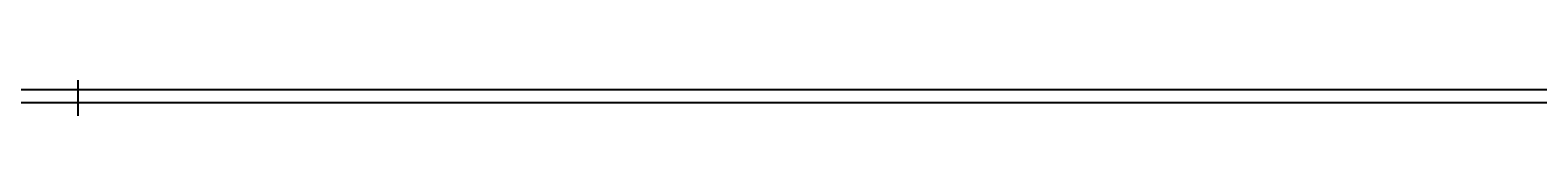
# Model space of a CAD drawing. Units: inches. Extents: x 35362 to 73946, y 43607 to 67532.
# Tile 101 of 134: x 50119 to 50761, y 49313 to 49320. Entities that reach past the tile are written whole.
import ezdxf

# ---------------------------------------------------------------- set-up
doc = ezdxf.new("R2010")
doc.units = ezdxf.units.IN
doc.header["$MEASUREMENT"] = 0
doc.layers.add('A-ANNO-DIMS', color=2, linetype='Continuous', lineweight=18)
doc.styles.get("Standard").update_dxf_attribs({"font": 'arial.ttf'})
doc.dimstyles.get("Standard").update_dxf_attribs({"dimtxt": 0.18, "dimasz": 0.18, "dimexe": 0.18, "dimexo": 0.0625, "dimgap": 0.09, "dimtad": 0, "dimtih": 1, "dimtoh": 1, "dimdec": 4, "dimzin": 0, "dimdsep": 46, "dimtxsty": 'Standard', "dimcen": 0.09, "dimadec": 0, "dimazin": 0, "dimtfac": 1, "dimtdec": 4, "dimtofl": 0, "dimtmove": 0, "dimatfit": 3, "dimfxl": 1, "dimtolj": 1, "dimtzin": 0, "dimarcsym": 0})

# ---------------------------------------------------------------- blocks, each defined once
blk = doc.blocks.new('*D11')
at = {"layer": 'A-ANNO-DIMS', "color": 0, "lineweight": -2, "transparency": 16777216}
for p, q in [((47978.66, 56028.77), (47978.66, 43606.68)), ((53109.76, 56028.77), (53109.76, 43606.68)), ((47978.84, 43606.86), (50543.87, 43606.86)), ((53109.58, 43606.86), (50544.55, 43606.86))]:
    blk.add_line(p, q, dxfattribs=at)
at = {"layer": 'A-ANNO-DIMS', "color": 0, "transparency": 16777216}
for points in [[(47978.84, 43606.89), (47978.84, 43606.83), (47978.66, 43606.86)], [(53109.58, 43606.89), (53109.58, 43606.83), (53109.76, 43606.86)]]:
    blk.add_solid(points, dxfattribs=at)
at = {"layer": 'Defpoints', "color": 0, "transparency": 16777216}
for p in [(47978.66, 56028.84), (53109.76, 56028.84), (53109.76, 43606.86)]:
    blk.add_point(p, dxfattribs=at)
at = {"layer": 'A-ANNO-DIMS', "color": 0, "transparency": 16777216, "insert": (50544.21, 43606.86), "char_height": 0.18, "attachment_point": 5}
blk.add_mtext('\\A1;5131', dxfattribs=at)
blk = doc.blocks.new('*D13')
at = {"layer": 'A-ANNO-DIMS', "color": 0, "lineweight": -2, "transparency": 16777216}
for p, q in [((48373.49, 51694.02), (48373.49, 43606.68)), ((51029.04, 51694.02), (51029.04, 43606.68)), ((48373.67, 43606.86), (49700.8, 43606.86)), ((51028.86, 43606.86), (49701.73, 43606.86))]:
    blk.add_line(p, q, dxfattribs=at)
at = {"layer": 'A-ANNO-DIMS', "color": 0, "transparency": 16777216}
for points in [[(48373.67, 43606.89), (48373.67, 43606.83), (48373.49, 43606.86)], [(51028.86, 43606.89), (51028.86, 43606.83), (51029.04, 43606.86)]]:
    blk.add_solid(points, dxfattribs=at)
at = {"layer": 'Defpoints', "color": 0, "transparency": 16777216}
for p in [(48373.49, 51694.09), (51029.04, 51694.09), (51029.04, 43606.86)]:
    blk.add_point(p, dxfattribs=at)
at = {"layer": 'A-ANNO-DIMS', "color": 0, "transparency": 16777216, "insert": (49701.27, 43606.86), "char_height": 0.18, "attachment_point": 5}
blk.add_mtext('\\A1;2655.6', dxfattribs=at)
blk = doc.blocks.new('*D17')
at = {"layer": 'A-ANNO-DIMS', "color": 0, "lineweight": -2, "transparency": 16777216}
for p, q in [((49923.31, 61293.22), (49923.31, 43606.68)), ((51913.93, 61293.22), (51913.93, 43606.68)), ((49923.49, 43606.86), (50918.16, 43606.86)), ((51913.75, 43606.86), (50919.07, 43606.86))]:
    blk.add_line(p, q, dxfattribs=at)
at = {"layer": 'A-ANNO-DIMS', "color": 0, "transparency": 16777216}
for points in [[(49923.49, 43606.89), (49923.49, 43606.83), (49923.31, 43606.86)], [(51913.75, 43606.89), (51913.75, 43606.83), (51913.93, 43606.86)]]:
    blk.add_solid(points, dxfattribs=at)
at = {"layer": 'Defpoints', "color": 0, "transparency": 16777216}
for p in [(49923.31, 61293.29), (51913.93, 61293.29), (51913.93, 43606.86)]:
    blk.add_point(p, dxfattribs=at)
at = {"layer": 'A-ANNO-DIMS', "color": 0, "transparency": 16777216, "insert": (50918.62, 43606.86), "char_height": 0.18, "attachment_point": 5}
blk.add_mtext('\\A1;1990.6', dxfattribs=at)
blk = doc.blocks.new('*D40')
at = {"layer": 'A-ANNO-DIMS', "color": 0, "lineweight": -2, "transparency": 16777216}
for p, q in [((56873.54, 53351.53), (35361.77, 53351.53)), ((35361.95, 53351.35), (35361.95, 51333.28)), ((35361.95, 49314.85), (35361.95, 51332.92)), ((51806.45, 49314.67), (35361.77, 49314.67))]:
    blk.add_line(p, q, dxfattribs=at)
at = {"layer": 'A-ANNO-DIMS', "color": 0, "transparency": 16777216}
for points in [[(35361.92, 53351.35), (35361.98, 53351.35), (35361.95, 53351.53)], [(35361.92, 49314.85), (35361.98, 49314.85), (35361.95, 49314.67)]]:
    blk.add_solid(points, dxfattribs=at)
at = {"layer": 'Defpoints', "color": 0, "transparency": 16777216}
for p in [(35361.95, 53351.53), (56873.6, 53351.53), (51806.52, 49314.67)]:
    blk.add_point(p, dxfattribs=at)
at = {"layer": 'A-ANNO-DIMS', "color": 0, "transparency": 16777216, "insert": (35361.95, 51333.1), "char_height": 0.18, "attachment_point": 5}
blk.add_mtext('\\A1;4036.9', dxfattribs=at)
blk = doc.blocks.new('*D67')
at = {"layer": 'A-ANNO-DIMS', "color": 0, "lineweight": -2, "transparency": 16777216}
for p, q in [((56873.54, 53351.53), (35361.77, 53351.53)), ((35361.95, 53351.35), (35361.95, 49400.89)), ((35361.95, 45450.07), (35361.95, 49400.53)), ((53793.58, 45449.89), (35361.77, 45449.89))]:
    blk.add_line(p, q, dxfattribs=at)
at = {"layer": 'A-ANNO-DIMS', "color": 0, "transparency": 16777216}
for points in [[(35361.92, 53351.35), (35361.98, 53351.35), (35361.95, 53351.53)], [(35361.92, 45450.07), (35361.98, 45450.07), (35361.95, 45449.89)]]:
    blk.add_solid(points, dxfattribs=at)
at = {"layer": 'Defpoints', "color": 0, "transparency": 16777216}
for p in [(35361.95, 53351.53), (56873.6, 53351.53), (53793.64, 45449.89)]:
    blk.add_point(p, dxfattribs=at)
at = {"layer": 'A-ANNO-DIMS', "color": 0, "transparency": 16777216, "insert": (35361.95, 49400.71), "char_height": 0.18, "attachment_point": 5}
blk.add_mtext('\\A1;7901.6', dxfattribs=at)
blk = doc.blocks.new('*D86')
at = {"layer": 'A-ANNO-DIMS', "color": 0, "lineweight": -2, "transparency": 16777216}
for p, q in [((51285.53, 49320.08), (35361.77, 49320.08)), ((35361.95, 49319.9), (35361.95, 49120.26)), ((35361.95, 48920.26), (35361.95, 49119.9)), ((51285.53, 48920.08), (35361.77, 48920.08))]:
    blk.add_line(p, q, dxfattribs=at)
at = {"layer": 'A-ANNO-DIMS', "color": 0, "transparency": 16777216}
for points in [[(35361.92, 49319.9), (35361.98, 49319.9), (35361.95, 49320.08)], [(35361.92, 48920.26), (35361.98, 48920.26), (35361.95, 48920.08)]]:
    blk.add_solid(points, dxfattribs=at)
at = {"layer": 'Defpoints', "color": 0, "transparency": 16777216}
for p in [(35361.95, 49320.08), (51285.59, 49320.08), (51285.59, 48920.08)]:
    blk.add_point(p, dxfattribs=at)
at = {"layer": 'A-ANNO-DIMS', "color": 0, "transparency": 16777216, "insert": (35361.95, 49120.08), "char_height": 0.18, "attachment_point": 5}
blk.add_mtext('\\A1;400.0', dxfattribs=at)
blk = doc.blocks.new('*D107')
at = {"layer": 'A-ANNO-DIMS', "color": 0, "lineweight": -2, "transparency": 16777216}
for p, q in [((50139.56, 59850.01), (50139.56, 43606.68)), ((51320.81, 59850.01), (51320.81, 43606.68)), ((50139.74, 43606.86), (50729.73, 43606.86)), ((51320.63, 43606.86), (50730.64, 43606.86))]:
    blk.add_line(p, q, dxfattribs=at)
at = {"layer": 'A-ANNO-DIMS', "color": 0, "transparency": 16777216}
for points in [[(50139.74, 43606.89), (50139.74, 43606.83), (50139.56, 43606.86)], [(51320.63, 43606.89), (51320.63, 43606.83), (51320.81, 43606.86)]]:
    blk.add_solid(points, dxfattribs=at)
at = {"layer": 'Defpoints', "color": 0, "transparency": 16777216}
for p in [(50139.56, 59850.08), (51320.81, 59850.08), (51320.81, 43606.86)]:
    blk.add_point(p, dxfattribs=at)
at = {"layer": 'A-ANNO-DIMS', "color": 0, "transparency": 16777216, "insert": (50730.19, 43606.86), "char_height": 0.18, "attachment_point": 5}
blk.add_mtext('\\A1;1181.3', dxfattribs=at)

msp = doc.modelspace()

# ---------------------------------------------------------------- dimensions: what is measured, and where the dimension line sits
at = {"layer": 'A-ANNO-DIMS'}
for base, p1, p2, override, picture, middle in [((51913.931, 43606.859), (49923.307, 61293.286), (51913.931, 61293.286), {"dimdec": 1, "dimlfac": 1, "dimrnd": 0, "dimzin": 0, "dimdsep": 46, "dimlunit": 2}, '*D17', (50918.619, 43606.859)), ((51320.8133, 43606.859), (50139.5627, 59850.0769), (51320.8133, 59850.0769), {"dimdec": 1, "dimlfac": 1, "dimrnd": 0, "dimzin": 0, "dimdsep": 46, "dimlunit": 2}, '*D107', (50730.188, 43606.859)), ((53109.76, 43606.859), (47978.665, 56028.836), (53109.76, 56028.836), {"dimdec": 0, "dimlfac": 1, "dimrnd": 0, "dimzin": 0, "dimdsep": 46, "dimlunit": 2}, '*D11', (50544.212, 43606.859)), ((51029.043, 43606.859), (48373.492, 51694.087), (51029.043, 51694.087), {"dimdec": 1, "dimlfac": 1, "dimrnd": 0, "dimzin": 0, "dimdsep": 46, "dimlunit": 2}, '*D13', (49701.267, 43606.859))]:
    dim = msp.add_linear_dim(base=base, p1=p1, p2=p2, dimstyle='Standard', override=override, dxfattribs=at)
    dim.commit()
    dim.dimension.update_dxf_attribs({"geometry": picture, "text_midpoint": middle})
for base, p1, p2, picture, middle in [((35361.949, 53351.529), (51806.517, 49314.669), (56873.602, 53351.529), '*D40', (35361.949, 51333.099)), ((35361.949, 53351.529), (53793.638, 45449.894), (56873.602, 53351.529), '*D67', (35361.949, 49400.712)), ((35361.949, 49320.079), (51285.595, 48920.079), (51285.595, 49320.079), '*D86', (35361.949, 49120.079))]:
    dim = msp.add_linear_dim(base=base, p1=p1, p2=p2, angle=90, dimstyle='Standard', override={"dimdec": 1, "dimlfac": 1, "dimrnd": 0, "dimzin": 0, "dimdsep": 46, "dimlunit": 2}, dxfattribs=at)
    dim.commit()
    dim.dimension.update_dxf_attribs({"geometry": picture, "text_midpoint": middle})

doc.saveas('drawing.dxf')
